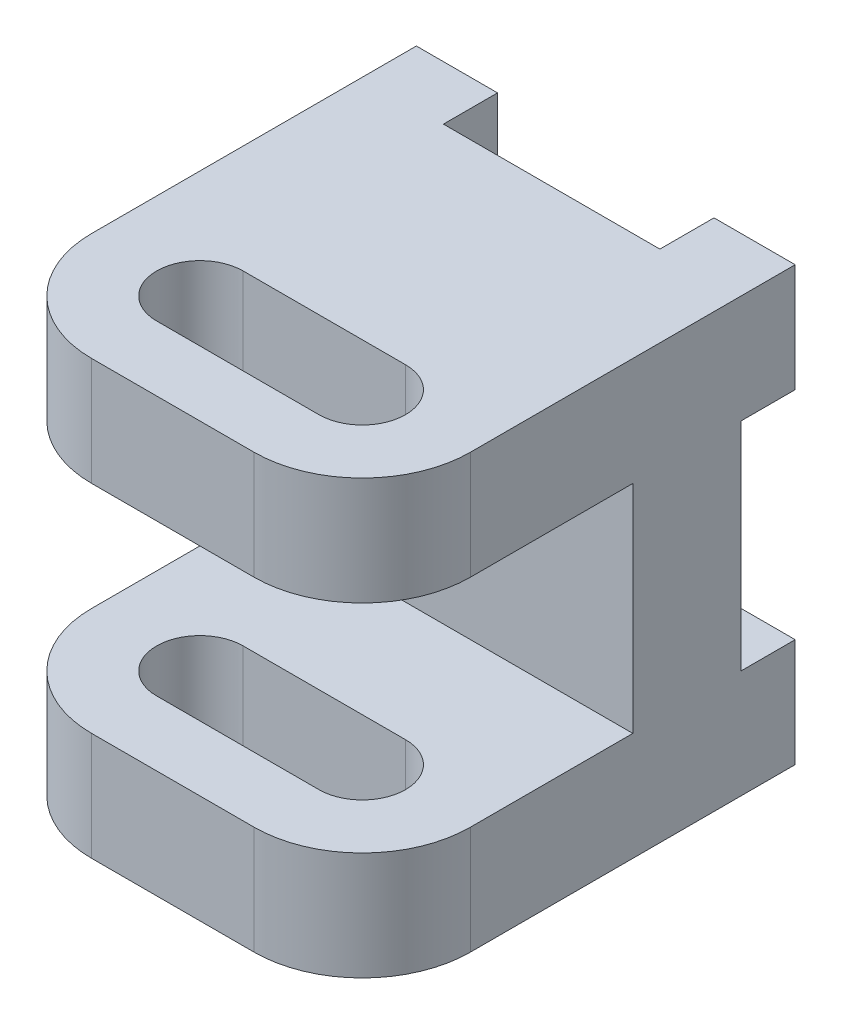
ISO-10303-21;
HEADER;
FILE_DESCRIPTION(('STEP AP214'),'2;1');
FILE_NAME('part.step','',(''),(''),'','','');
FILE_SCHEMA(('AUTOMOTIVE_DESIGN { 1 0 10303 214 1 1 1 1 }'));
ENDSEC;
DATA;
#1=APPLICATION_CONTEXT('core data for automotive mechanical design processes');
#2=APPLICATION_PROTOCOL_DEFINITION('international standard','automotive_design',2000,#1);
#3=PRODUCT_CONTEXT('',#1,'mechanical');
#4=PRODUCT('Part','Part','',(#3));
#5=PRODUCT_RELATED_PRODUCT_CATEGORY('part','',(#4));
#6=PRODUCT_DEFINITION_FORMATION('','',#4);
#7=PRODUCT_DEFINITION_CONTEXT('part definition',#1,'design');
#8=PRODUCT_DEFINITION('design','',#6,#7);
#9=PRODUCT_DEFINITION_SHAPE('','',#8);
#10=(LENGTH_UNIT() NAMED_UNIT(*) SI_UNIT(.MILLI.,.METRE.));
#11=(NAMED_UNIT(*) PLANE_ANGLE_UNIT() SI_UNIT($,.RADIAN.));
#12=(NAMED_UNIT(*) SI_UNIT($,.STERADIAN.) SOLID_ANGLE_UNIT());
#13=UNCERTAINTY_MEASURE_WITH_UNIT(LENGTH_MEASURE(1.E-05),#10,'distance_accuracy_value','');
#14=(GEOMETRIC_REPRESENTATION_CONTEXT(3) GLOBAL_UNCERTAINTY_ASSIGNED_CONTEXT((#13)) GLOBAL_UNIT_ASSIGNED_CONTEXT((#10,
#11,#12)) REPRESENTATION_CONTEXT('',''));
#15=CARTESIAN_POINT('',(0.,0.,0.));
#16=DIRECTION('',(0.,0.,1.));
#17=DIRECTION('',(1.,0.,0.));
#18=AXIS2_PLACEMENT_3D('',#15,#16,#17);
#19=CARTESIAN_POINT('',(0.,0.,20.));
#20=DIRECTION('',(0.,0.,1.));
#21=DIRECTION('',(1.,0.,0.));
#22=AXIS2_PLACEMENT_3D('',#19,#20,#21);
#23=PLANE('',#22);
#24=DIRECTION('',(0.,1.,0.));
#25=VECTOR('',#24,1.);
#26=CARTESIAN_POINT('',(70.,0.,20.));
#27=LINE('',#26,#25);
#28=CARTESIAN_POINT('',(70.,15.,20.));
#29=VERTEX_POINT('',#28);
#30=CARTESIAN_POINT('',(70.,55.,20.));
#31=VERTEX_POINT('',#30);
#32=EDGE_CURVE('E483',#29,#31,#27,.T.);
#33=ORIENTED_EDGE('',*,*,#32,.T.);
#34=DIRECTION('',(-1.,0.,0.));
#35=VECTOR('',#34,1.);
#36=CARTESIAN_POINT('',(0.,55.,20.));
#37=LINE('',#36,#35);
#38=CARTESIAN_POINT('',(0.,55.,20.));
#39=VERTEX_POINT('',#38);
#40=EDGE_CURVE('E312',#31,#39,#37,.T.);
#41=ORIENTED_EDGE('',*,*,#40,.T.);
#42=DIRECTION('',(0.,-1.,0.));
#43=VECTOR('',#42,1.);
#44=CARTESIAN_POINT('',(0.,70.,20.));
#45=LINE('',#44,#43);
#46=CARTESIAN_POINT('',(0.,15.,20.));
#47=VERTEX_POINT('',#46);
#48=EDGE_CURVE('E485',#39,#47,#45,.T.);
#49=ORIENTED_EDGE('',*,*,#48,.T.);
#50=DIRECTION('',(1.,0.,0.));
#51=VECTOR('',#50,1.);
#52=CARTESIAN_POINT('',(70.,15.,20.));
#53=LINE('',#52,#51);
#54=EDGE_CURVE('E361',#47,#29,#53,.T.);
#55=ORIENTED_EDGE('',*,*,#54,.T.);
#56=EDGE_LOOP('',(#33,#41,#49,#55));
#57=FACE_BOUND('',#56,.T.);
#58=ADVANCED_FACE('F44',(#57),#23,.T.);
#59=CARTESIAN_POINT('',(0.,0.,0.));
#60=DIRECTION('',(0.,0.,1.));
#61=DIRECTION('',(1.,0.,0.));
#62=AXIS2_PLACEMENT_3D('',#59,#60,#61);
#63=PLANE('',#62);
#64=DIRECTION('',(1.,0.,0.));
#65=VECTOR('',#64,1.);
#66=CARTESIAN_POINT('',(0.,15.,0.));
#67=LINE('',#66,#65);
#68=CARTESIAN_POINT('',(55.,15.,0.));
#69=VERTEX_POINT('',#68);
#70=CARTESIAN_POINT('',(70.,15.,0.));
#71=VERTEX_POINT('',#70);
#72=EDGE_CURVE('E427',#69,#71,#67,.T.);
#73=ORIENTED_EDGE('',*,*,#72,.F.);
#74=DIRECTION('',(0.,-1.,0.));
#75=VECTOR('',#74,1.);
#76=CARTESIAN_POINT('',(55.,25.,0.));
#77=LINE('',#76,#75);
#78=CARTESIAN_POINT('',(55.,-5.,0.));
#79=VERTEX_POINT('',#78);
#80=EDGE_CURVE('E467',#69,#79,#77,.T.);
#81=ORIENTED_EDGE('',*,*,#80,.T.);
#82=DIRECTION('',(1.,0.,0.));
#83=VECTOR('',#82,1.);
#84=CARTESIAN_POINT('',(55.,-5.,0.));
#85=LINE('',#84,#83);
#86=CARTESIAN_POINT('',(15.,-5.,0.));
#87=VERTEX_POINT('',#86);
#88=EDGE_CURVE('E412',#87,#79,#85,.T.);
#89=ORIENTED_EDGE('',*,*,#88,.F.);
#90=DIRECTION('',(0.,-1.,0.));
#91=VECTOR('',#90,1.);
#92=CARTESIAN_POINT('',(15.,25.,0.));
#93=LINE('',#92,#91);
#94=CARTESIAN_POINT('',(15.,15.,0.));
#95=VERTEX_POINT('',#94);
#96=EDGE_CURVE('E478',#95,#87,#93,.T.);
#97=ORIENTED_EDGE('',*,*,#96,.F.);
#98=CARTESIAN_POINT('',(0.,15.,0.));
#99=VERTEX_POINT('',#98);
#100=EDGE_CURVE('E440',#99,#95,#67,.T.);
#101=ORIENTED_EDGE('',*,*,#100,.F.);
#102=DIRECTION('',(0.,-1.,0.));
#103=VECTOR('',#102,1.);
#104=CARTESIAN_POINT('',(0.,70.,0.));
#105=LINE('',#104,#103);
#106=CARTESIAN_POINT('',(0.,55.,0.));
#107=VERTEX_POINT('',#106);
#108=EDGE_CURVE('E476',#107,#99,#105,.T.);
#109=ORIENTED_EDGE('',*,*,#108,.F.);
#110=DIRECTION('',(1.,0.,0.));
#111=VECTOR('',#110,1.);
#112=CARTESIAN_POINT('',(0.,55.,0.));
#113=LINE('',#112,#111);
#114=CARTESIAN_POINT('',(15.,55.,0.));
#115=VERTEX_POINT('',#114);
#116=EDGE_CURVE('E450',#107,#115,#113,.T.);
#117=ORIENTED_EDGE('',*,*,#116,.T.);
#118=DIRECTION('',(0.,1.,0.));
#119=VECTOR('',#118,1.);
#120=CARTESIAN_POINT('',(15.,45.,0.));
#121=LINE('',#120,#119);
#122=CARTESIAN_POINT('',(15.,75.,0.));
#123=VERTEX_POINT('',#122);
#124=EDGE_CURVE('E457',#115,#123,#121,.T.);
#125=ORIENTED_EDGE('',*,*,#124,.T.);
#126=DIRECTION('',(-1.,0.,0.));
#127=VECTOR('',#126,1.);
#128=CARTESIAN_POINT('',(55.,75.,0.));
#129=LINE('',#128,#127);
#130=CARTESIAN_POINT('',(55.,75.,0.));
#131=VERTEX_POINT('',#130);
#132=EDGE_CURVE('E400',#131,#123,#129,.T.);
#133=ORIENTED_EDGE('',*,*,#132,.F.);
#134=DIRECTION('',(0.,1.,0.));
#135=VECTOR('',#134,1.);
#136=CARTESIAN_POINT('',(55.,45.,0.));
#137=LINE('',#136,#135);
#138=CARTESIAN_POINT('',(55.,55.,0.));
#139=VERTEX_POINT('',#138);
#140=EDGE_CURVE('E456',#139,#131,#137,.T.);
#141=ORIENTED_EDGE('',*,*,#140,.F.);
#142=CARTESIAN_POINT('',(70.,55.,0.));
#143=VERTEX_POINT('',#142);
#144=EDGE_CURVE('E452',#139,#143,#113,.T.);
#145=ORIENTED_EDGE('',*,*,#144,.T.);
#146=DIRECTION('',(0.,1.,0.));
#147=VECTOR('',#146,1.);
#148=CARTESIAN_POINT('',(70.,0.,0.));
#149=LINE('',#148,#147);
#150=EDGE_CURVE('E484',#71,#143,#149,.T.);
#151=ORIENTED_EDGE('',*,*,#150,.F.);
#152=EDGE_LOOP('',(#73,#81,#89,#97,#101,#109,#117,#125,#133,#141,#145,#151));
#153=FACE_BOUND('',#152,.T.);
#154=ADVANCED_FACE('F520',(#153),#63,.F.);
#155=CARTESIAN_POINT('',(0.,70.,20.));
#156=DIRECTION('',(1.,0.,0.));
#157=DIRECTION('',(0.,0.,-1.));
#158=AXIS2_PLACEMENT_3D('',#155,#156,#157);
#159=PLANE('',#158);
#160=ORIENTED_EDGE('',*,*,#108,.T.);
#161=DIRECTION('',(0.,0.,-1.));
#162=VECTOR('',#161,1.);
#163=CARTESIAN_POINT('',(0.,15.,0.));
#164=LINE('',#163,#162);
#165=CARTESIAN_POINT('',(0.,15.,-10.));
#166=VERTEX_POINT('',#165);
#167=EDGE_CURVE('E430',#99,#166,#164,.T.);
#168=ORIENTED_EDGE('',*,*,#167,.T.);
#169=DIRECTION('',(0.,-1.,0.));
#170=VECTOR('',#169,1.);
#171=CARTESIAN_POINT('',(0.,25.,-10.));
#172=LINE('',#171,#170);
#173=CARTESIAN_POINT('',(0.,-5.,-10.));
#174=VERTEX_POINT('',#173);
#175=EDGE_CURVE('E475',#166,#174,#172,.T.);
#176=ORIENTED_EDGE('',*,*,#175,.T.);
#177=DIRECTION('',(0.,0.,-1.));
#178=VECTOR('',#177,1.);
#179=CARTESIAN_POINT('',(0.,-5.,-10.));
#180=LINE('',#179,#178);
#181=CARTESIAN_POINT('',(0.,-5.,49.9999999999999));
#182=VERTEX_POINT('',#181);
#183=EDGE_CURVE('E407',#182,#174,#180,.T.);
#184=ORIENTED_EDGE('',*,*,#183,.F.);
#185=DIRECTION('',(0.,-1.,0.));
#186=VECTOR('',#185,1.);
#187=CARTESIAN_POINT('',(0.,15.,49.9999999999999));
#188=LINE('',#187,#186);
#189=CARTESIAN_POINT('',(0.,15.,49.9999999999999));
#190=VERTEX_POINT('',#189);
#191=EDGE_CURVE('E382',#190,#182,#188,.T.);
#192=ORIENTED_EDGE('',*,*,#191,.F.);
#193=DIRECTION('',(0.,0.,-1.));
#194=VECTOR('',#193,1.);
#195=CARTESIAN_POINT('',(0.,15.,20.));
#196=LINE('',#195,#194);
#197=EDGE_CURVE('E359',#190,#47,#196,.T.);
#198=ORIENTED_EDGE('',*,*,#197,.T.);
#199=ORIENTED_EDGE('',*,*,#48,.F.);
#200=DIRECTION('',(0.,0.,1.));
#201=VECTOR('',#200,1.);
#202=CARTESIAN_POINT('',(0.,55.,20.));
#203=LINE('',#202,#201);
#204=CARTESIAN_POINT('',(0.,55.,49.9999999999999));
#205=VERTEX_POINT('',#204);
#206=EDGE_CURVE('E317',#39,#205,#203,.T.);
#207=ORIENTED_EDGE('',*,*,#206,.T.);
#208=DIRECTION('',(0.,1.,0.));
#209=VECTOR('',#208,1.);
#210=CARTESIAN_POINT('',(0.,55.,49.9999999999999));
#211=LINE('',#210,#209);
#212=CARTESIAN_POINT('',(0.,75.,49.9999999999999));
#213=VERTEX_POINT('',#212);
#214=EDGE_CURVE('E335',#205,#213,#211,.T.);
#215=ORIENTED_EDGE('',*,*,#214,.T.);
#216=DIRECTION('',(0.,0.,1.));
#217=VECTOR('',#216,1.);
#218=CARTESIAN_POINT('',(0.,75.,-10.));
#219=LINE('',#218,#217);
#220=CARTESIAN_POINT('',(0.,75.,-10.));
#221=VERTEX_POINT('',#220);
#222=EDGE_CURVE('E379',#221,#213,#219,.T.);
#223=ORIENTED_EDGE('',*,*,#222,.F.);
#224=DIRECTION('',(0.,1.,0.));
#225=VECTOR('',#224,1.);
#226=CARTESIAN_POINT('',(0.,45.,-10.));
#227=LINE('',#226,#225);
#228=CARTESIAN_POINT('',(0.,55.,-10.));
#229=VERTEX_POINT('',#228);
#230=EDGE_CURVE('E463',#229,#221,#227,.T.);
#231=ORIENTED_EDGE('',*,*,#230,.F.);
#232=DIRECTION('',(0.,0.,1.));
#233=VECTOR('',#232,1.);
#234=CARTESIAN_POINT('',(0.,55.,0.));
#235=LINE('',#234,#233);
#236=EDGE_CURVE('E441',#229,#107,#235,.T.);
#237=ORIENTED_EDGE('',*,*,#236,.T.);
#238=EDGE_LOOP('',(#160,#168,#176,#184,#192,#198,#199,#207,#215,#223,#231,#237));
#239=FACE_BOUND('',#238,.T.);
#240=ADVANCED_FACE('F50',(#239),#159,.F.);
#241=CARTESIAN_POINT('',(70.,0.,20.));
#242=DIRECTION('',(-1.,0.,0.));
#243=DIRECTION('',(0.,0.,1.));
#244=AXIS2_PLACEMENT_3D('',#241,#242,#243);
#245=PLANE('',#244);
#246=DIRECTION('',(0.,-1.,0.));
#247=VECTOR('',#246,1.);
#248=CARTESIAN_POINT('',(70.,25.,-10.));
#249=LINE('',#248,#247);
#250=CARTESIAN_POINT('',(70.,15.,-10.));
#251=VERTEX_POINT('',#250);
#252=CARTESIAN_POINT('',(70.,-5.,-10.));
#253=VERTEX_POINT('',#252);
#254=EDGE_CURVE('E468',#251,#253,#249,.T.);
#255=ORIENTED_EDGE('',*,*,#254,.F.);
#256=DIRECTION('',(0.,0.,-1.));
#257=VECTOR('',#256,1.);
#258=CARTESIAN_POINT('',(70.,15.,0.));
#259=LINE('',#258,#257);
#260=EDGE_CURVE('E428',#71,#251,#259,.T.);
#261=ORIENTED_EDGE('',*,*,#260,.F.);
#262=ORIENTED_EDGE('',*,*,#150,.T.);
#263=DIRECTION('',(0.,0.,1.));
#264=VECTOR('',#263,1.);
#265=CARTESIAN_POINT('',(70.,55.,0.));
#266=LINE('',#265,#264);
#267=CARTESIAN_POINT('',(70.,55.,-10.));
#268=VERTEX_POINT('',#267);
#269=EDGE_CURVE('E439',#268,#143,#266,.T.);
#270=ORIENTED_EDGE('',*,*,#269,.F.);
#271=DIRECTION('',(0.,1.,0.));
#272=VECTOR('',#271,1.);
#273=CARTESIAN_POINT('',(70.,45.,-10.));
#274=LINE('',#273,#272);
#275=CARTESIAN_POINT('',(70.,75.,-10.));
#276=VERTEX_POINT('',#275);
#277=EDGE_CURVE('E460',#268,#276,#274,.T.);
#278=ORIENTED_EDGE('',*,*,#277,.T.);
#279=DIRECTION('',(0.,0.,-1.));
#280=VECTOR('',#279,1.);
#281=CARTESIAN_POINT('',(70.,75.,20.));
#282=LINE('',#281,#280);
#283=CARTESIAN_POINT('',(70.,75.,49.9999999999999));
#284=VERTEX_POINT('',#283);
#285=EDGE_CURVE('E389',#284,#276,#282,.T.);
#286=ORIENTED_EDGE('',*,*,#285,.F.);
#287=DIRECTION('',(0.,1.,0.));
#288=VECTOR('',#287,1.);
#289=CARTESIAN_POINT('',(70.,55.,49.9999999999999));
#290=LINE('',#289,#288);
#291=CARTESIAN_POINT('',(70.,55.,49.9999999999999));
#292=VERTEX_POINT('',#291);
#293=EDGE_CURVE('E338',#292,#284,#290,.T.);
#294=ORIENTED_EDGE('',*,*,#293,.F.);
#295=DIRECTION('',(0.,0.,-1.));
#296=VECTOR('',#295,1.);
#297=CARTESIAN_POINT('',(70.,55.,20.));
#298=LINE('',#297,#296);
#299=EDGE_CURVE('E329',#292,#31,#298,.T.);
#300=ORIENTED_EDGE('',*,*,#299,.T.);
#301=ORIENTED_EDGE('',*,*,#32,.F.);
#302=DIRECTION('',(0.,0.,1.));
#303=VECTOR('',#302,1.);
#304=CARTESIAN_POINT('',(70.,15.,49.9999999999999));
#305=LINE('',#304,#303);
#306=CARTESIAN_POINT('',(70.,15.,49.9999999999999));
#307=VERTEX_POINT('',#306);
#308=EDGE_CURVE('E366',#29,#307,#305,.T.);
#309=ORIENTED_EDGE('',*,*,#308,.T.);
#310=DIRECTION('',(0.,-1.,0.));
#311=VECTOR('',#310,1.);
#312=CARTESIAN_POINT('',(70.,15.,49.9999999999999));
#313=LINE('',#312,#311);
#314=CARTESIAN_POINT('',(70.,-5.,49.9999999999999));
#315=VERTEX_POINT('',#314);
#316=EDGE_CURVE('E380',#307,#315,#313,.T.);
#317=ORIENTED_EDGE('',*,*,#316,.T.);
#318=DIRECTION('',(0.,0.,1.));
#319=VECTOR('',#318,1.);
#320=CARTESIAN_POINT('',(70.,-5.,20.));
#321=LINE('',#320,#319);
#322=EDGE_CURVE('E425',#253,#315,#321,.T.);
#323=ORIENTED_EDGE('',*,*,#322,.F.);
#324=EDGE_LOOP('',(#255,#261,#262,#270,#278,#286,#294,#300,#301,#309,#317,#323));
#325=FACE_BOUND('',#324,.T.);
#326=ADVANCED_FACE('F529',(#325),#245,.F.);
#327=CARTESIAN_POINT('',(15.,25.,0.));
#328=DIRECTION('',(1.,0.,0.));
#329=DIRECTION('',(0.,0.,-1.));
#330=AXIS2_PLACEMENT_3D('',#327,#328,#329);
#331=PLANE('',#330);
#332=DIRECTION('',(0.,0.,-1.));
#333=VECTOR('',#332,1.);
#334=CARTESIAN_POINT('',(15.,15.,0.));
#335=LINE('',#334,#333);
#336=CARTESIAN_POINT('',(15.,15.,-10.));
#337=VERTEX_POINT('',#336);
#338=EDGE_CURVE('E434',#95,#337,#335,.T.);
#339=ORIENTED_EDGE('',*,*,#338,.F.);
#340=ORIENTED_EDGE('',*,*,#96,.T.);
#341=DIRECTION('',(0.,0.,1.));
#342=VECTOR('',#341,1.);
#343=CARTESIAN_POINT('',(15.,-5.,0.));
#344=LINE('',#343,#342);
#345=CARTESIAN_POINT('',(15.,-5.,-10.));
#346=VERTEX_POINT('',#345);
#347=EDGE_CURVE('E415',#346,#87,#344,.T.);
#348=ORIENTED_EDGE('',*,*,#347,.F.);
#349=DIRECTION('',(0.,-1.,0.));
#350=VECTOR('',#349,1.);
#351=CARTESIAN_POINT('',(15.,25.,-10.));
#352=LINE('',#351,#350);
#353=EDGE_CURVE('E479',#337,#346,#352,.T.);
#354=ORIENTED_EDGE('',*,*,#353,.F.);
#355=EDGE_LOOP('',(#339,#340,#348,#354));
#356=FACE_BOUND('',#355,.T.);
#357=ADVANCED_FACE('F535',(#356),#331,.T.);
#358=CARTESIAN_POINT('',(15.,25.,-10.));
#359=DIRECTION('',(0.,0.,-1.));
#360=DIRECTION('',(-1.,0.,0.));
#361=AXIS2_PLACEMENT_3D('',#358,#359,#360);
#362=PLANE('',#361);
#363=DIRECTION('',(1.,0.,0.));
#364=VECTOR('',#363,1.);
#365=CARTESIAN_POINT('',(0.,15.,-10.));
#366=LINE('',#365,#364);
#367=EDGE_CURVE('E435',#166,#337,#366,.T.);
#368=ORIENTED_EDGE('',*,*,#367,.T.);
#369=ORIENTED_EDGE('',*,*,#353,.T.);
#370=DIRECTION('',(1.,0.,0.));
#371=VECTOR('',#370,1.);
#372=CARTESIAN_POINT('',(15.,-5.,-10.));
#373=LINE('',#372,#371);
#374=EDGE_CURVE('E406',#174,#346,#373,.T.);
#375=ORIENTED_EDGE('',*,*,#374,.F.);
#376=ORIENTED_EDGE('',*,*,#175,.F.);
#377=EDGE_LOOP('',(#368,#369,#375,#376));
#378=FACE_BOUND('',#377,.T.);
#379=ADVANCED_FACE('F527',(#378),#362,.T.);
#380=CARTESIAN_POINT('',(55.,25.,-10.));
#381=DIRECTION('',(0.,0.,-1.));
#382=DIRECTION('',(-1.,0.,0.));
#383=AXIS2_PLACEMENT_3D('',#380,#381,#382);
#384=PLANE('',#383);
#385=CARTESIAN_POINT('',(55.,15.,-10.));
#386=VERTEX_POINT('',#385);
#387=EDGE_CURVE('E436',#386,#251,#366,.T.);
#388=ORIENTED_EDGE('',*,*,#387,.T.);
#389=ORIENTED_EDGE('',*,*,#254,.T.);
#390=DIRECTION('',(1.,0.,0.));
#391=VECTOR('',#390,1.);
#392=CARTESIAN_POINT('',(70.,-5.,-10.));
#393=LINE('',#392,#391);
#394=CARTESIAN_POINT('',(55.,-5.,-10.));
#395=VERTEX_POINT('',#394);
#396=EDGE_CURVE('E423',#395,#253,#393,.T.);
#397=ORIENTED_EDGE('',*,*,#396,.F.);
#398=DIRECTION('',(0.,-1.,0.));
#399=VECTOR('',#398,1.);
#400=CARTESIAN_POINT('',(55.,25.,-10.));
#401=LINE('',#400,#399);
#402=EDGE_CURVE('E474',#386,#395,#401,.T.);
#403=ORIENTED_EDGE('',*,*,#402,.F.);
#404=EDGE_LOOP('',(#388,#389,#397,#403));
#405=FACE_BOUND('',#404,.T.);
#406=ADVANCED_FACE('F546',(#405),#384,.T.);
#407=CARTESIAN_POINT('',(55.,25.,0.));
#408=DIRECTION('',(-1.,0.,0.));
#409=DIRECTION('',(0.,0.,1.));
#410=AXIS2_PLACEMENT_3D('',#407,#408,#409);
#411=PLANE('',#410);
#412=DIRECTION('',(0.,0.,1.));
#413=VECTOR('',#412,1.);
#414=CARTESIAN_POINT('',(55.,15.,0.));
#415=LINE('',#414,#413);
#416=EDGE_CURVE('E486',#386,#69,#415,.T.);
#417=ORIENTED_EDGE('',*,*,#416,.F.);
#418=ORIENTED_EDGE('',*,*,#402,.T.);
#419=DIRECTION('',(0.,0.,-1.));
#420=VECTOR('',#419,1.);
#421=CARTESIAN_POINT('',(55.,-5.,-10.));
#422=LINE('',#421,#420);
#423=EDGE_CURVE('E417',#79,#395,#422,.T.);
#424=ORIENTED_EDGE('',*,*,#423,.F.);
#425=ORIENTED_EDGE('',*,*,#80,.F.);
#426=EDGE_LOOP('',(#417,#418,#424,#425));
#427=FACE_BOUND('',#426,.T.);
#428=ADVANCED_FACE('F554',(#427),#411,.T.);
#429=CARTESIAN_POINT('',(0.,45.,-10.));
#430=DIRECTION('',(0.,0.,-1.));
#431=DIRECTION('',(-1.,0.,0.));
#432=AXIS2_PLACEMENT_3D('',#429,#430,#431);
#433=PLANE('',#432);
#434=DIRECTION('',(1.,0.,0.));
#435=VECTOR('',#434,1.);
#436=CARTESIAN_POINT('',(0.,55.,-10.));
#437=LINE('',#436,#435);
#438=CARTESIAN_POINT('',(15.,55.,-10.));
#439=VERTEX_POINT('',#438);
#440=EDGE_CURVE('E455',#229,#439,#437,.T.);
#441=ORIENTED_EDGE('',*,*,#440,.F.);
#442=ORIENTED_EDGE('',*,*,#230,.T.);
#443=DIRECTION('',(-1.,0.,0.));
#444=VECTOR('',#443,1.);
#445=CARTESIAN_POINT('',(15.,75.,-10.));
#446=LINE('',#445,#444);
#447=CARTESIAN_POINT('',(15.,75.,-10.));
#448=VERTEX_POINT('',#447);
#449=EDGE_CURVE('E401',#448,#221,#446,.T.);
#450=ORIENTED_EDGE('',*,*,#449,.F.);
#451=DIRECTION('',(0.,1.,0.));
#452=VECTOR('',#451,1.);
#453=CARTESIAN_POINT('',(15.,45.,-10.));
#454=LINE('',#453,#452);
#455=EDGE_CURVE('E470',#439,#448,#454,.T.);
#456=ORIENTED_EDGE('',*,*,#455,.F.);
#457=EDGE_LOOP('',(#441,#442,#450,#456));
#458=FACE_BOUND('',#457,.T.);
#459=ADVANCED_FACE('F581',(#458),#433,.T.);
#460=CARTESIAN_POINT('',(15.,45.,0.));
#461=DIRECTION('',(1.,0.,0.));
#462=DIRECTION('',(0.,0.,-1.));
#463=AXIS2_PLACEMENT_3D('',#460,#461,#462);
#464=PLANE('',#463);
#465=DIRECTION('',(0.,0.,1.));
#466=VECTOR('',#465,1.);
#467=CARTESIAN_POINT('',(15.,55.,0.));
#468=LINE('',#467,#466);
#469=EDGE_CURVE('E453',#439,#115,#468,.T.);
#470=ORIENTED_EDGE('',*,*,#469,.F.);
#471=ORIENTED_EDGE('',*,*,#455,.T.);
#472=DIRECTION('',(0.,0.,-1.));
#473=VECTOR('',#472,1.);
#474=CARTESIAN_POINT('',(15.,75.,0.));
#475=LINE('',#474,#473);
#476=EDGE_CURVE('E399',#123,#448,#475,.T.);
#477=ORIENTED_EDGE('',*,*,#476,.F.);
#478=ORIENTED_EDGE('',*,*,#124,.F.);
#479=EDGE_LOOP('',(#470,#471,#477,#478));
#480=FACE_BOUND('',#479,.T.);
#481=ADVANCED_FACE('F578',(#480),#464,.T.);
#482=CARTESIAN_POINT('',(55.,45.,0.));
#483=DIRECTION('',(-1.,0.,0.));
#484=DIRECTION('',(0.,0.,1.));
#485=AXIS2_PLACEMENT_3D('',#482,#483,#484);
#486=PLANE('',#485);
#487=DIRECTION('',(0.,0.,-1.));
#488=VECTOR('',#487,1.);
#489=CARTESIAN_POINT('',(55.,55.,0.));
#490=LINE('',#489,#488);
#491=CARTESIAN_POINT('',(55.,55.,-10.));
#492=VERTEX_POINT('',#491);
#493=EDGE_CURVE('E448',#139,#492,#490,.T.);
#494=ORIENTED_EDGE('',*,*,#493,.F.);
#495=ORIENTED_EDGE('',*,*,#140,.T.);
#496=DIRECTION('',(0.,0.,1.));
#497=VECTOR('',#496,1.);
#498=CARTESIAN_POINT('',(55.,75.,-10.));
#499=LINE('',#498,#497);
#500=CARTESIAN_POINT('',(55.,75.,-10.));
#501=VERTEX_POINT('',#500);
#502=EDGE_CURVE('E394',#501,#131,#499,.T.);
#503=ORIENTED_EDGE('',*,*,#502,.F.);
#504=DIRECTION('',(0.,1.,0.));
#505=VECTOR('',#504,1.);
#506=CARTESIAN_POINT('',(55.,45.,-10.));
#507=LINE('',#506,#505);
#508=EDGE_CURVE('E461',#492,#501,#507,.T.);
#509=ORIENTED_EDGE('',*,*,#508,.F.);
#510=EDGE_LOOP('',(#494,#495,#503,#509));
#511=FACE_BOUND('',#510,.T.);
#512=ADVANCED_FACE('F573',(#511),#486,.T.);
#513=CARTESIAN_POINT('',(55.,45.,-10.));
#514=DIRECTION('',(0.,0.,-1.));
#515=DIRECTION('',(-1.,0.,0.));
#516=AXIS2_PLACEMENT_3D('',#513,#514,#515);
#517=PLANE('',#516);
#518=EDGE_CURVE('E443',#492,#268,#437,.T.);
#519=ORIENTED_EDGE('',*,*,#518,.F.);
#520=ORIENTED_EDGE('',*,*,#508,.T.);
#521=DIRECTION('',(-1.,0.,0.));
#522=VECTOR('',#521,1.);
#523=CARTESIAN_POINT('',(70.,75.,-10.));
#524=LINE('',#523,#522);
#525=EDGE_CURVE('E393',#276,#501,#524,.T.);
#526=ORIENTED_EDGE('',*,*,#525,.F.);
#527=ORIENTED_EDGE('',*,*,#277,.F.);
#528=EDGE_LOOP('',(#519,#520,#526,#527));
#529=FACE_BOUND('',#528,.T.);
#530=ADVANCED_FACE('F568',(#529),#517,.T.);
#531=CARTESIAN_POINT('',(0.,55.,0.));
#532=DIRECTION('',(0.,1.,0.));
#533=DIRECTION('',(0.,0.,1.));
#534=AXIS2_PLACEMENT_3D('',#531,#532,#533);
#535=PLANE('',#534);
#536=ORIENTED_EDGE('',*,*,#493,.T.);
#537=ORIENTED_EDGE('',*,*,#518,.T.);
#538=ORIENTED_EDGE('',*,*,#269,.T.);
#539=ORIENTED_EDGE('',*,*,#144,.F.);
#540=EDGE_LOOP('',(#536,#537,#538,#539));
#541=FACE_BOUND('',#540,.T.);
#542=ADVANCED_FACE('F634',(#541),#535,.F.);
#543=ORIENTED_EDGE('',*,*,#469,.T.);
#544=ORIENTED_EDGE('',*,*,#116,.F.);
#545=ORIENTED_EDGE('',*,*,#236,.F.);
#546=ORIENTED_EDGE('',*,*,#440,.T.);
#547=EDGE_LOOP('',(#543,#544,#545,#546));
#548=FACE_BOUND('',#547,.T.);
#549=ADVANCED_FACE('F632',(#548),#535,.F.);
#550=CARTESIAN_POINT('',(0.,15.,0.));
#551=DIRECTION('',(0.,-1.,0.));
#552=DIRECTION('',(0.,0.,-1.));
#553=AXIS2_PLACEMENT_3D('',#550,#551,#552);
#554=PLANE('',#553);
#555=ORIENTED_EDGE('',*,*,#416,.T.);
#556=ORIENTED_EDGE('',*,*,#72,.T.);
#557=ORIENTED_EDGE('',*,*,#260,.T.);
#558=ORIENTED_EDGE('',*,*,#387,.F.);
#559=EDGE_LOOP('',(#555,#556,#557,#558));
#560=FACE_BOUND('',#559,.T.);
#561=ADVANCED_FACE('F559',(#560),#554,.F.);
#562=ORIENTED_EDGE('',*,*,#338,.T.);
#563=ORIENTED_EDGE('',*,*,#367,.F.);
#564=ORIENTED_EDGE('',*,*,#167,.F.);
#565=ORIENTED_EDGE('',*,*,#100,.T.);
#566=EDGE_LOOP('',(#562,#563,#564,#565));
#567=FACE_BOUND('',#566,.T.);
#568=ADVANCED_FACE('F629',(#567),#554,.F.);
#569=CARTESIAN_POINT('',(0.,-5.,0.));
#570=DIRECTION('',(0.,1.,0.));
#571=DIRECTION('',(0.,0.,1.));
#572=AXIS2_PLACEMENT_3D('',#569,#570,#571);
#573=PLANE('',#572);
#574=DIRECTION('',(1.,0.,0.));
#575=VECTOR('',#574,1.);
#576=CARTESIAN_POINT('',(20.0000000000001,-5.,42.));
#577=LINE('',#576,#575);
#578=CARTESIAN_POINT('',(20.0000000000001,-5.,42.));
#579=VERTEX_POINT('',#578);
#580=CARTESIAN_POINT('',(49.9999999999999,-5.,42.));
#581=VERTEX_POINT('',#580);
#582=EDGE_CURVE('E290',#579,#581,#577,.T.);
#583=ORIENTED_EDGE('',*,*,#582,.F.);
#584=CARTESIAN_POINT('',(20.0000000000001,-5.,50.));
#585=DIRECTION('',(0.,-1.,0.));
#586=DIRECTION('',(0.,0.,-1.));
#587=AXIS2_PLACEMENT_3D('',#584,#585,#586);
#588=CIRCLE('',#587,8.);
#589=CARTESIAN_POINT('',(20.0000000000001,-5.,58.));
#590=VERTEX_POINT('',#589);
#591=EDGE_CURVE('E58',#590,#579,#588,.T.);
#592=ORIENTED_EDGE('',*,*,#591,.F.);
#593=DIRECTION('',(-1.,0.,0.));
#594=VECTOR('',#593,1.);
#595=CARTESIAN_POINT('',(20.0000000000001,-5.,58.));
#596=LINE('',#595,#594);
#597=CARTESIAN_POINT('',(49.9999999999999,-5.,58.));
#598=VERTEX_POINT('',#597);
#599=EDGE_CURVE('E279',#598,#590,#596,.T.);
#600=ORIENTED_EDGE('',*,*,#599,.F.);
#601=CARTESIAN_POINT('',(49.9999999999999,-5.,50.));
#602=DIRECTION('',(0.,-1.,0.));
#603=DIRECTION('',(0.,0.,-1.));
#604=AXIS2_PLACEMENT_3D('',#601,#602,#603);
#605=CIRCLE('',#604,8.);
#606=EDGE_CURVE('E283',#581,#598,#605,.T.);
#607=ORIENTED_EDGE('',*,*,#606,.F.);
#608=EDGE_LOOP('',(#583,#592,#600,#607));
#609=FACE_BOUND('',#608,.T.);
#610=ORIENTED_EDGE('',*,*,#183,.T.);
#611=ORIENTED_EDGE('',*,*,#374,.T.);
#612=ORIENTED_EDGE('',*,*,#347,.T.);
#613=ORIENTED_EDGE('',*,*,#88,.T.);
#614=ORIENTED_EDGE('',*,*,#423,.T.);
#615=ORIENTED_EDGE('',*,*,#396,.T.);
#616=ORIENTED_EDGE('',*,*,#322,.T.);
#617=CARTESIAN_POINT('',(50.,-5.,50.));
#618=DIRECTION('',(0.,-1.,0.));
#619=DIRECTION('',(0.,0.,-1.));
#620=AXIS2_PLACEMENT_3D('',#617,#618,#619);
#621=CIRCLE('',#620,20.);
#622=CARTESIAN_POINT('',(49.9999999999999,-5.,70.));
#623=VERTEX_POINT('',#622);
#624=EDGE_CURVE('E344',#315,#623,#621,.T.);
#625=ORIENTED_EDGE('',*,*,#624,.T.);
#626=DIRECTION('',(-1.,0.,0.));
#627=VECTOR('',#626,1.);
#628=CARTESIAN_POINT('',(20.0000000000001,-5.,70.));
#629=LINE('',#628,#627);
#630=CARTESIAN_POINT('',(20.0000000000001,-5.,70.));
#631=VERTEX_POINT('',#630);
#632=EDGE_CURVE('E375',#623,#631,#629,.T.);
#633=ORIENTED_EDGE('',*,*,#632,.T.);
#634=CARTESIAN_POINT('',(20.,-5.,50.));
#635=DIRECTION('',(0.,-1.,0.));
#636=DIRECTION('',(0.,0.,-1.));
#637=AXIS2_PLACEMENT_3D('',#634,#635,#636);
#638=CIRCLE('',#637,20.);
#639=EDGE_CURVE('E353',#631,#182,#638,.T.);
#640=ORIENTED_EDGE('',*,*,#639,.T.);
#641=EDGE_LOOP('',(#610,#611,#612,#613,#614,#615,#616,#625,#633,#640));
#642=FACE_BOUND('',#641,.T.);
#643=ADVANCED_FACE('F548',(#609,#642),#573,.F.);
#644=CARTESIAN_POINT('',(0.,75.,0.));
#645=DIRECTION('',(0.,1.,0.));
#646=DIRECTION('',(0.,0.,1.));
#647=AXIS2_PLACEMENT_3D('',#644,#645,#646);
#648=PLANE('',#647);
#649=CARTESIAN_POINT('',(20.0000000000001,75.,50.));
#650=DIRECTION('',(0.,-1.,0.));
#651=DIRECTION('',(0.,0.,-1.));
#652=AXIS2_PLACEMENT_3D('',#649,#650,#651);
#653=CIRCLE('',#652,8.);
#654=CARTESIAN_POINT('',(20.0000000000001,75.,58.));
#655=VERTEX_POINT('',#654);
#656=CARTESIAN_POINT('',(20.0000000000001,75.,42.));
#657=VERTEX_POINT('',#656);
#658=EDGE_CURVE('E263',#655,#657,#653,.T.);
#659=ORIENTED_EDGE('',*,*,#658,.T.);
#660=DIRECTION('',(1.,0.,0.));
#661=VECTOR('',#660,1.);
#662=CARTESIAN_POINT('',(20.0000000000001,75.,42.));
#663=LINE('',#662,#661);
#664=CARTESIAN_POINT('',(49.9999999999999,75.,42.));
#665=VERTEX_POINT('',#664);
#666=EDGE_CURVE('E268',#657,#665,#663,.T.);
#667=ORIENTED_EDGE('',*,*,#666,.T.);
#668=CARTESIAN_POINT('',(49.9999999999999,75.,50.));
#669=DIRECTION('',(0.,-1.,0.));
#670=DIRECTION('',(0.,0.,-1.));
#671=AXIS2_PLACEMENT_3D('',#668,#669,#670);
#672=CIRCLE('',#671,8.);
#673=CARTESIAN_POINT('',(49.9999999999999,75.,58.));
#674=VERTEX_POINT('',#673);
#675=EDGE_CURVE('E66',#665,#674,#672,.T.);
#676=ORIENTED_EDGE('',*,*,#675,.T.);
#677=DIRECTION('',(-1.,0.,0.));
#678=VECTOR('',#677,1.);
#679=CARTESIAN_POINT('',(20.0000000000001,75.,58.));
#680=LINE('',#679,#678);
#681=EDGE_CURVE('E280',#674,#655,#680,.T.);
#682=ORIENTED_EDGE('',*,*,#681,.T.);
#683=EDGE_LOOP('',(#659,#667,#676,#682));
#684=FACE_BOUND('',#683,.T.);
#685=ORIENTED_EDGE('',*,*,#222,.T.);
#686=CARTESIAN_POINT('',(20.,75.,50.));
#687=DIRECTION('',(0.,1.,0.));
#688=DIRECTION('',(0.,0.,1.));
#689=AXIS2_PLACEMENT_3D('',#686,#687,#688);
#690=CIRCLE('',#689,20.);
#691=CARTESIAN_POINT('',(20.,75.,70.));
#692=VERTEX_POINT('',#691);
#693=EDGE_CURVE('E315',#213,#692,#690,.T.);
#694=ORIENTED_EDGE('',*,*,#693,.T.);
#695=DIRECTION('',(1.,0.,0.));
#696=VECTOR('',#695,1.);
#697=CARTESIAN_POINT('',(20.0000000000001,75.,70.));
#698=LINE('',#697,#696);
#699=CARTESIAN_POINT('',(49.9999999999999,75.,70.));
#700=VERTEX_POINT('',#699);
#701=EDGE_CURVE('E334',#692,#700,#698,.T.);
#702=ORIENTED_EDGE('',*,*,#701,.T.);
#703=CARTESIAN_POINT('',(50.,75.,50.));
#704=DIRECTION('',(0.,1.,0.));
#705=DIRECTION('',(0.,0.,1.));
#706=AXIS2_PLACEMENT_3D('',#703,#704,#705);
#707=CIRCLE('',#706,20.);
#708=EDGE_CURVE('E320',#700,#284,#707,.T.);
#709=ORIENTED_EDGE('',*,*,#708,.T.);
#710=ORIENTED_EDGE('',*,*,#285,.T.);
#711=ORIENTED_EDGE('',*,*,#525,.T.);
#712=ORIENTED_EDGE('',*,*,#502,.T.);
#713=ORIENTED_EDGE('',*,*,#132,.T.);
#714=ORIENTED_EDGE('',*,*,#476,.T.);
#715=ORIENTED_EDGE('',*,*,#449,.T.);
#716=EDGE_LOOP('',(#685,#694,#702,#709,#710,#711,#712,#713,#714,#715));
#717=FACE_BOUND('',#716,.T.);
#718=ADVANCED_FACE('F274',(#684,#717),#648,.T.);
#719=CARTESIAN_POINT('',(50.,15.,50.));
#720=DIRECTION('',(0.,-1.,0.));
#721=DIRECTION('',(0.,0.,-1.));
#722=AXIS2_PLACEMENT_3D('',#719,#720,#721);
#723=CYLINDRICAL_SURFACE('',#722,20.);
#724=ORIENTED_EDGE('',*,*,#624,.F.);
#725=ORIENTED_EDGE('',*,*,#316,.F.);
#726=CARTESIAN_POINT('',(50.,15.,50.));
#727=DIRECTION('',(0.,-1.,0.));
#728=DIRECTION('',(0.,0.,-1.));
#729=AXIS2_PLACEMENT_3D('',#726,#727,#728);
#730=CIRCLE('',#729,20.);
#731=CARTESIAN_POINT('',(49.9999999999999,15.,70.));
#732=VERTEX_POINT('',#731);
#733=EDGE_CURVE('E347',#307,#732,#730,.T.);
#734=ORIENTED_EDGE('',*,*,#733,.T.);
#735=DIRECTION('',(0.,-1.,0.));
#736=VECTOR('',#735,1.);
#737=CARTESIAN_POINT('',(49.9999999999999,15.,70.));
#738=LINE('',#737,#736);
#739=EDGE_CURVE('E367',#732,#623,#738,.T.);
#740=ORIENTED_EDGE('',*,*,#739,.T.);
#741=EDGE_LOOP('',(#724,#725,#734,#740));
#742=FACE_BOUND('',#741,.T.);
#743=ADVANCED_FACE('F617',(#742),#723,.T.);
#744=CARTESIAN_POINT('',(20.,15.,50.));
#745=DIRECTION('',(0.,-1.,0.));
#746=DIRECTION('',(0.,0.,-1.));
#747=AXIS2_PLACEMENT_3D('',#744,#745,#746);
#748=CYLINDRICAL_SURFACE('',#747,20.);
#749=ORIENTED_EDGE('',*,*,#639,.F.);
#750=DIRECTION('',(0.,-1.,0.));
#751=VECTOR('',#750,1.);
#752=CARTESIAN_POINT('',(20.0000000000001,15.,70.));
#753=LINE('',#752,#751);
#754=CARTESIAN_POINT('',(20.0000000000001,15.,70.));
#755=VERTEX_POINT('',#754);
#756=EDGE_CURVE('E381',#755,#631,#753,.T.);
#757=ORIENTED_EDGE('',*,*,#756,.F.);
#758=CARTESIAN_POINT('',(20.,15.,50.));
#759=DIRECTION('',(0.,-1.,0.));
#760=DIRECTION('',(0.,0.,-1.));
#761=AXIS2_PLACEMENT_3D('',#758,#759,#760);
#762=CIRCLE('',#761,20.);
#763=EDGE_CURVE('E357',#755,#190,#762,.T.);
#764=ORIENTED_EDGE('',*,*,#763,.T.);
#765=ORIENTED_EDGE('',*,*,#191,.T.);
#766=EDGE_LOOP('',(#749,#757,#764,#765));
#767=FACE_BOUND('',#766,.T.);
#768=ADVANCED_FACE('F607',(#767),#748,.T.);
#769=CARTESIAN_POINT('',(20.0000000000001,15.,70.));
#770=DIRECTION('',(0.,0.,1.));
#771=DIRECTION('',(1.,0.,0.));
#772=AXIS2_PLACEMENT_3D('',#769,#770,#771);
#773=PLANE('',#772);
#774=ORIENTED_EDGE('',*,*,#632,.F.);
#775=ORIENTED_EDGE('',*,*,#739,.F.);
#776=DIRECTION('',(-1.,0.,0.));
#777=VECTOR('',#776,1.);
#778=CARTESIAN_POINT('',(20.0000000000001,15.,70.));
#779=LINE('',#778,#777);
#780=EDGE_CURVE('E352',#732,#755,#779,.T.);
#781=ORIENTED_EDGE('',*,*,#780,.T.);
#782=ORIENTED_EDGE('',*,*,#756,.T.);
#783=EDGE_LOOP('',(#774,#775,#781,#782));
#784=FACE_BOUND('',#783,.T.);
#785=ADVANCED_FACE('F613',(#784),#773,.T.);
#786=CARTESIAN_POINT('',(50.,15.,50.));
#787=DIRECTION('',(0.,-1.,0.));
#788=DIRECTION('',(0.,0.,-1.));
#789=AXIS2_PLACEMENT_3D('',#786,#787,#788);
#790=PLANE('',#789);
#791=DIRECTION('',(-1.,0.,0.));
#792=VECTOR('',#791,1.);
#793=CARTESIAN_POINT('',(50.,15.,58.));
#794=LINE('',#793,#792);
#795=CARTESIAN_POINT('',(49.9999999999999,15.,58.));
#796=VERTEX_POINT('',#795);
#797=CARTESIAN_POINT('',(20.0000000000001,15.,58.));
#798=VERTEX_POINT('',#797);
#799=EDGE_CURVE('E306',#796,#798,#794,.T.);
#800=ORIENTED_EDGE('',*,*,#799,.T.);
#801=CARTESIAN_POINT('',(20.0000000000001,15.,50.));
#802=DIRECTION('',(0.,-1.,0.));
#803=DIRECTION('',(0.,0.,-1.));
#804=AXIS2_PLACEMENT_3D('',#801,#802,#803);
#805=CIRCLE('',#804,8.);
#806=CARTESIAN_POINT('',(20.0000000000001,15.,42.));
#807=VERTEX_POINT('',#806);
#808=EDGE_CURVE('E307',#798,#807,#805,.T.);
#809=ORIENTED_EDGE('',*,*,#808,.T.);
#810=DIRECTION('',(1.,0.,0.));
#811=VECTOR('',#810,1.);
#812=CARTESIAN_POINT('',(50.,15.,42.));
#813=LINE('',#812,#811);
#814=CARTESIAN_POINT('',(49.9999999999999,15.,42.));
#815=VERTEX_POINT('',#814);
#816=EDGE_CURVE('E295',#807,#815,#813,.T.);
#817=ORIENTED_EDGE('',*,*,#816,.T.);
#818=CARTESIAN_POINT('',(49.9999999999999,15.,50.));
#819=DIRECTION('',(0.,-1.,0.));
#820=DIRECTION('',(0.,0.,-1.));
#821=AXIS2_PLACEMENT_3D('',#818,#819,#820);
#822=CIRCLE('',#821,8.);
#823=EDGE_CURVE('E303',#815,#796,#822,.T.);
#824=ORIENTED_EDGE('',*,*,#823,.T.);
#825=EDGE_LOOP('',(#800,#809,#817,#824));
#826=FACE_BOUND('',#825,.T.);
#827=ORIENTED_EDGE('',*,*,#733,.F.);
#828=ORIENTED_EDGE('',*,*,#308,.F.);
#829=ORIENTED_EDGE('',*,*,#54,.F.);
#830=ORIENTED_EDGE('',*,*,#197,.F.);
#831=ORIENTED_EDGE('',*,*,#763,.F.);
#832=ORIENTED_EDGE('',*,*,#780,.F.);
#833=EDGE_LOOP('',(#827,#828,#829,#830,#831,#832));
#834=FACE_BOUND('',#833,.T.);
#835=ADVANCED_FACE('F608',(#826,#834),#790,.F.);
#836=CARTESIAN_POINT('',(50.,55.,50.));
#837=DIRECTION('',(0.,1.,0.));
#838=DIRECTION('',(0.,0.,1.));
#839=AXIS2_PLACEMENT_3D('',#836,#837,#838);
#840=CYLINDRICAL_SURFACE('',#839,20.);
#841=ORIENTED_EDGE('',*,*,#708,.F.);
#842=DIRECTION('',(0.,1.,0.));
#843=VECTOR('',#842,1.);
#844=CARTESIAN_POINT('',(49.9999999999999,55.,70.));
#845=LINE('',#844,#843);
#846=CARTESIAN_POINT('',(49.9999999999999,55.,70.));
#847=VERTEX_POINT('',#846);
#848=EDGE_CURVE('E341',#847,#700,#845,.T.);
#849=ORIENTED_EDGE('',*,*,#848,.F.);
#850=CARTESIAN_POINT('',(50.,55.,50.));
#851=DIRECTION('',(0.,1.,0.));
#852=DIRECTION('',(0.,0.,1.));
#853=AXIS2_PLACEMENT_3D('',#850,#851,#852);
#854=CIRCLE('',#853,20.);
#855=EDGE_CURVE('E328',#847,#292,#854,.T.);
#856=ORIENTED_EDGE('',*,*,#855,.T.);
#857=ORIENTED_EDGE('',*,*,#293,.T.);
#858=EDGE_LOOP('',(#841,#849,#856,#857));
#859=FACE_BOUND('',#858,.T.);
#860=ADVANCED_FACE('F599',(#859),#840,.T.);
#861=CARTESIAN_POINT('',(20.0000000000001,55.,70.));
#862=DIRECTION('',(0.,0.,1.));
#863=DIRECTION('',(1.,0.,0.));
#864=AXIS2_PLACEMENT_3D('',#861,#862,#863);
#865=PLANE('',#864);
#866=ORIENTED_EDGE('',*,*,#701,.F.);
#867=DIRECTION('',(0.,1.,0.));
#868=VECTOR('',#867,1.);
#869=CARTESIAN_POINT('',(20.,55.,70.));
#870=LINE('',#869,#868);
#871=CARTESIAN_POINT('',(20.,55.,70.));
#872=VERTEX_POINT('',#871);
#873=EDGE_CURVE('E348',#872,#692,#870,.T.);
#874=ORIENTED_EDGE('',*,*,#873,.F.);
#875=DIRECTION('',(1.,0.,0.));
#876=VECTOR('',#875,1.);
#877=CARTESIAN_POINT('',(20.0000000000001,55.,70.));
#878=LINE('',#877,#876);
#879=EDGE_CURVE('E324',#872,#847,#878,.T.);
#880=ORIENTED_EDGE('',*,*,#879,.T.);
#881=ORIENTED_EDGE('',*,*,#848,.T.);
#882=EDGE_LOOP('',(#866,#874,#880,#881));
#883=FACE_BOUND('',#882,.T.);
#884=ADVANCED_FACE('F594',(#883),#865,.T.);
#885=CARTESIAN_POINT('',(20.,55.,50.));
#886=DIRECTION('',(0.,1.,0.));
#887=DIRECTION('',(0.,0.,1.));
#888=AXIS2_PLACEMENT_3D('',#885,#886,#887);
#889=CYLINDRICAL_SURFACE('',#888,20.);
#890=ORIENTED_EDGE('',*,*,#693,.F.);
#891=ORIENTED_EDGE('',*,*,#214,.F.);
#892=CARTESIAN_POINT('',(20.,55.,50.));
#893=DIRECTION('',(0.,1.,0.));
#894=DIRECTION('',(0.,0.,1.));
#895=AXIS2_PLACEMENT_3D('',#892,#893,#894);
#896=CIRCLE('',#895,20.);
#897=EDGE_CURVE('E318',#205,#872,#896,.T.);
#898=ORIENTED_EDGE('',*,*,#897,.T.);
#899=ORIENTED_EDGE('',*,*,#873,.T.);
#900=EDGE_LOOP('',(#890,#891,#898,#899));
#901=FACE_BOUND('',#900,.T.);
#902=ADVANCED_FACE('F591',(#901),#889,.T.);
#903=CARTESIAN_POINT('',(50.,55.,50.));
#904=DIRECTION('',(0.,1.,0.));
#905=DIRECTION('',(0.,0.,1.));
#906=AXIS2_PLACEMENT_3D('',#903,#904,#905);
#907=PLANE('',#906);
#908=DIRECTION('',(-1.,0.,0.));
#909=VECTOR('',#908,1.);
#910=CARTESIAN_POINT('',(50.,55.,42.));
#911=LINE('',#910,#909);
#912=CARTESIAN_POINT('',(49.9999999999999,55.,42.));
#913=VERTEX_POINT('',#912);
#914=CARTESIAN_POINT('',(20.0000000000001,55.,42.));
#915=VERTEX_POINT('',#914);
#916=EDGE_CURVE('E495',#913,#915,#911,.T.);
#917=ORIENTED_EDGE('',*,*,#916,.T.);
#918=CARTESIAN_POINT('',(20.0000000000001,55.,50.));
#919=DIRECTION('',(0.,1.,0.));
#920=DIRECTION('',(0.,0.,1.));
#921=AXIS2_PLACEMENT_3D('',#918,#919,#920);
#922=CIRCLE('',#921,8.);
#923=CARTESIAN_POINT('',(20.0000000000001,55.,58.));
#924=VERTEX_POINT('',#923);
#925=EDGE_CURVE('E11',#915,#924,#922,.T.);
#926=ORIENTED_EDGE('',*,*,#925,.T.);
#927=DIRECTION('',(1.,0.,0.));
#928=VECTOR('',#927,1.);
#929=CARTESIAN_POINT('',(50.,55.,58.));
#930=LINE('',#929,#928);
#931=CARTESIAN_POINT('',(49.9999999999999,55.,58.));
#932=VERTEX_POINT('',#931);
#933=EDGE_CURVE('E52',#924,#932,#930,.T.);
#934=ORIENTED_EDGE('',*,*,#933,.T.);
#935=CARTESIAN_POINT('',(49.9999999999999,55.,50.));
#936=DIRECTION('',(0.,1.,0.));
#937=DIRECTION('',(0.,0.,1.));
#938=AXIS2_PLACEMENT_3D('',#935,#936,#937);
#939=CIRCLE('',#938,8.);
#940=EDGE_CURVE('E494',#932,#913,#939,.T.);
#941=ORIENTED_EDGE('',*,*,#940,.T.);
#942=EDGE_LOOP('',(#917,#926,#934,#941));
#943=FACE_BOUND('',#942,.T.);
#944=ORIENTED_EDGE('',*,*,#40,.F.);
#945=ORIENTED_EDGE('',*,*,#299,.F.);
#946=ORIENTED_EDGE('',*,*,#855,.F.);
#947=ORIENTED_EDGE('',*,*,#879,.F.);
#948=ORIENTED_EDGE('',*,*,#897,.F.);
#949=ORIENTED_EDGE('',*,*,#206,.F.);
#950=EDGE_LOOP('',(#944,#945,#946,#947,#948,#949));
#951=FACE_BOUND('',#950,.T.);
#952=ADVANCED_FACE('F498',(#943,#951),#907,.F.);
#953=CARTESIAN_POINT('',(20.0000000000001,75.,42.));
#954=DIRECTION('',(0.,0.,-1.));
#955=DIRECTION('',(-1.,0.,0.));
#956=AXIS2_PLACEMENT_3D('',#953,#954,#955);
#957=PLANE('',#956);
#958=DIRECTION('',(0.,-1.,0.));
#959=VECTOR('',#958,1.);
#960=CARTESIAN_POINT('',(49.9999999999999,75.,42.));
#961=LINE('',#960,#959);
#962=EDGE_CURVE('E272',#665,#913,#961,.T.);
#963=ORIENTED_EDGE('',*,*,#962,.F.);
#964=ORIENTED_EDGE('',*,*,#666,.F.);
#965=DIRECTION('',(0.,-1.,0.));
#966=VECTOR('',#965,1.);
#967=CARTESIAN_POINT('',(20.0000000000001,75.,42.));
#968=LINE('',#967,#966);
#969=EDGE_CURVE('E257',#657,#915,#968,.T.);
#970=ORIENTED_EDGE('',*,*,#969,.T.);
#971=ORIENTED_EDGE('',*,*,#916,.F.);
#972=EDGE_LOOP('',(#963,#964,#970,#971));
#973=FACE_BOUND('',#972,.T.);
#974=ADVANCED_FACE('F269',(#973),#957,.F.);
#975=CARTESIAN_POINT('',(49.9999999999999,75.,50.));
#976=DIRECTION('',(0.,-1.,0.));
#977=DIRECTION('',(0.,0.,-1.));
#978=AXIS2_PLACEMENT_3D('',#975,#976,#977);
#979=CYLINDRICAL_SURFACE('',#978,8.);
#980=DIRECTION('',(0.,-1.,0.));
#981=VECTOR('',#980,1.);
#982=CARTESIAN_POINT('',(49.9999999999999,75.,58.));
#983=LINE('',#982,#981);
#984=EDGE_CURVE('E298',#674,#932,#983,.T.);
#985=ORIENTED_EDGE('',*,*,#984,.F.);
#986=ORIENTED_EDGE('',*,*,#675,.F.);
#987=ORIENTED_EDGE('',*,*,#962,.T.);
#988=ORIENTED_EDGE('',*,*,#940,.F.);
#989=EDGE_LOOP('',(#985,#986,#987,#988));
#990=FACE_BOUND('',#989,.T.);
#991=ADVANCED_FACE('F505',(#990),#979,.F.);
#992=CARTESIAN_POINT('',(20.0000000000001,75.,58.));
#993=DIRECTION('',(0.,0.,1.));
#994=DIRECTION('',(1.,0.,0.));
#995=AXIS2_PLACEMENT_3D('',#992,#993,#994);
#996=PLANE('',#995);
#997=DIRECTION('',(0.,-1.,0.));
#998=VECTOR('',#997,1.);
#999=CARTESIAN_POINT('',(20.0000000000001,75.,58.));
#1000=LINE('',#999,#998);
#1001=EDGE_CURVE('E292',#655,#924,#1000,.T.);
#1002=ORIENTED_EDGE('',*,*,#1001,.F.);
#1003=ORIENTED_EDGE('',*,*,#681,.F.);
#1004=ORIENTED_EDGE('',*,*,#984,.T.);
#1005=ORIENTED_EDGE('',*,*,#933,.F.);
#1006=EDGE_LOOP('',(#1002,#1003,#1004,#1005));
#1007=FACE_BOUND('',#1006,.T.);
#1008=ADVANCED_FACE('F501',(#1007),#996,.F.);
#1009=CARTESIAN_POINT('',(20.0000000000001,75.,50.));
#1010=DIRECTION('',(0.,-1.,0.));
#1011=DIRECTION('',(0.,0.,-1.));
#1012=AXIS2_PLACEMENT_3D('',#1009,#1010,#1011);
#1013=CYLINDRICAL_SURFACE('',#1012,8.);
#1014=ORIENTED_EDGE('',*,*,#969,.F.);
#1015=ORIENTED_EDGE('',*,*,#658,.F.);
#1016=ORIENTED_EDGE('',*,*,#1001,.T.);
#1017=ORIENTED_EDGE('',*,*,#925,.F.);
#1018=EDGE_LOOP('',(#1014,#1015,#1016,#1017));
#1019=FACE_BOUND('',#1018,.T.);
#1020=ADVANCED_FACE('F259',(#1019),#1013,.F.);
#1021=EDGE_CURVE('E294',#798,#590,#1000,.T.);
#1022=ORIENTED_EDGE('',*,*,#1021,.T.);
#1023=ORIENTED_EDGE('',*,*,#591,.T.);
#1024=EDGE_CURVE('E266',#807,#579,#968,.T.);
#1025=ORIENTED_EDGE('',*,*,#1024,.F.);
#1026=ORIENTED_EDGE('',*,*,#808,.F.);
#1027=EDGE_LOOP('',(#1022,#1023,#1025,#1026));
#1028=FACE_BOUND('',#1027,.T.);
#1029=ADVANCED_FACE('F775',(#1028),#1013,.F.);
#1030=EDGE_CURVE('E299',#796,#598,#983,.T.);
#1031=ORIENTED_EDGE('',*,*,#1030,.T.);
#1032=ORIENTED_EDGE('',*,*,#599,.T.);
#1033=ORIENTED_EDGE('',*,*,#1021,.F.);
#1034=ORIENTED_EDGE('',*,*,#799,.F.);
#1035=EDGE_LOOP('',(#1031,#1032,#1033,#1034));
#1036=FACE_BOUND('',#1035,.T.);
#1037=ADVANCED_FACE('F512',(#1036),#996,.F.);
#1038=EDGE_CURVE('E262',#815,#581,#961,.T.);
#1039=ORIENTED_EDGE('',*,*,#1038,.T.);
#1040=ORIENTED_EDGE('',*,*,#606,.T.);
#1041=ORIENTED_EDGE('',*,*,#1030,.F.);
#1042=ORIENTED_EDGE('',*,*,#823,.F.);
#1043=EDGE_LOOP('',(#1039,#1040,#1041,#1042));
#1044=FACE_BOUND('',#1043,.T.);
#1045=ADVANCED_FACE('F504',(#1044),#979,.F.);
#1046=ORIENTED_EDGE('',*,*,#1024,.T.);
#1047=ORIENTED_EDGE('',*,*,#582,.T.);
#1048=ORIENTED_EDGE('',*,*,#1038,.F.);
#1049=ORIENTED_EDGE('',*,*,#816,.F.);
#1050=EDGE_LOOP('',(#1046,#1047,#1048,#1049));
#1051=FACE_BOUND('',#1050,.T.);
#1052=ADVANCED_FACE('F514',(#1051),#957,.F.);
#1053=CLOSED_SHELL('',(#58,#154,#240,#326,#357,#379,#406,#428,#459,#481,#512,#530,#542,#549,
#561,#568,#643,#718,#743,#768,#785,#835,#860,#884,#902,#952,#974,#991,#1008,#1020,#1029,#1037,
#1045,#1052));
#1054=MANIFOLD_SOLID_BREP('B2',#1053);
#1055=ADVANCED_BREP_SHAPE_REPRESENTATION('',(#18,#1054),#14);
#1056=SHAPE_DEFINITION_REPRESENTATION(#9,#1055);
ENDSEC;
END-ISO-10303-21;
